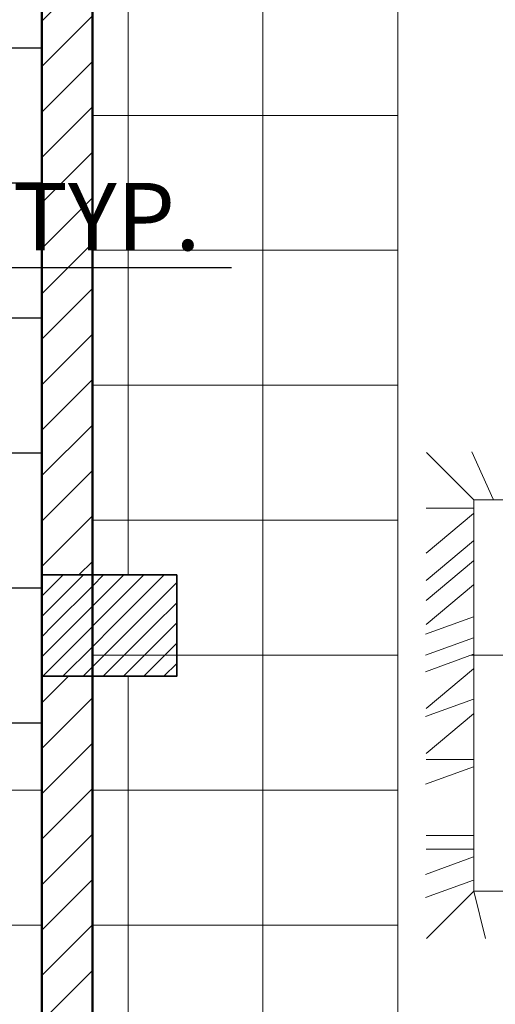
# Model space of a CAD drawing. Units: millimetres. Extents: x 225995 to 227247, y 225507 to 226008.
# Tile 5 of 23: x 226378 to 226421, y 225780 to 225867. Entities that reach past the tile are written whole.
import ezdxf

# ---------------------------------------------------------------- set-up
doc = ezdxf.new("R2010")
doc.units = ezdxf.units.MM
for name, color, linetype, lineweight in [('A-ANNO-DIMS', 2, 'Continuous', 18), ('A-COLS', 40, 'Continuous', 35), ('A-FLOR-PATT', 8, 'Continuous', 13), ('A-FLOR-STRS', 141, 'Continuous', 25), ('A-FURN', 9, 'Continuous', 18), ('A-WALL', 7, 'Continuous', 50), ('A-WALL-PATT', 8, 'Continuous', 13)]:
    doc.layers.add(name, color=color, linetype=linetype, lineweight=lineweight)
doc.styles.get("Standard").update_dxf_attribs({"font": 'arial.ttf'})
doc.dimstyles.new('ISO-25', dxfattribs={"dimtxt": 6, "dimasz": 2.5, "dimexe": 1.25, "dimexo": 0.625, "dimtad": 1, "dimdec": 0, "dimlunit": 3, "dimtxsty": 'Standard', "dimcen": 2.5, "dimadec": 0, "dimazin": 0, "dimtfac": 1, "dimtdec": 0, "dimtmove": 0, "dimatfit": 3, "dimfxl": 1, "dimarcsym": 0})
pattern_1 = [(45, (0, 118.1362), (-0.898025612, 0.898025612), [])]

# ---------------------------------------------------------------- blocks, each defined once
blk = doc.blocks.new('A$C6D2A2628')
for p, q in [((0.1019, 0.9267), (0.0019, 1.0267)), ((0.0977, 1.0278), (0.1431, 0.9278)), ((0.291, 0.9267), (0.1019, 0.9267)), ((0.1019, 0.9267), (0.1019, 0.1)), ((0.0015, 0.9091), (0.1015, 0.9091)), ((0.0015, 0.8141), (0.1015, 0.8978)), ((0.0015, 0.7564), (0.1015, 0.84)), ((0.0015, 0.7139), (0.1015, 0.7975)), ((0.0015, 0.6633), (0.1015, 0.7469)), ((0, 0.6428), (0.1015, 0.6794)), ((0, 0.5984), (0.1015, 0.6351)), ((0, 0.5636), (0.1015, 0.6003)), ((0.0015, 0.4859), (0.1015, 0.5695)), ((0, 0.4686), (0.1015, 0.5053)), ((0.0015, 0.3909), (0.1015, 0.4745)), ((0.0015, 0.3783), (0.1015, 0.3783)), ((0, 0.3261), (0.1015, 0.3628)), ((0.0015, 0.2173), (0.1015, 0.2173)), ((0.0015, 0.1884), (0.1015, 0.1884)), ((0, 0.1355), (0.1015, 0.1722)), ((0, 0.0863), (0.1015, 0.1229)), ((0.1019, 0.1), (0.0019, 0)), ((0.1019, 0.1), (1.9932, 0.1)), ((0.1019, 0.1), (0.1266, 0))]:
    blk.add_line(p, q)
blk = doc.blocks.new('*D81')
at = {"layer": 'A-ANNO-DIMS', "color": 0, "lineweight": -2, "transparency": 16777216}
for p, q in [((226280.276, 225843.99), (226280.276, 225846.51)), ((226292.912, 225843.99), (226292.912, 225846.51)), ((226282.776, 225845.26), (226290.412, 225845.26)), ((226292.912, 225845.26), (226397.254, 225845.26))]:
    blk.add_line(p, q, dxfattribs=at)
at = {"layer": 'A-ANNO-DIMS', "color": 0, "transparency": 16777216}
for points in [[(226282.776, 225845.677), (226282.776, 225844.844), (226280.276, 225845.26)], [(226290.412, 225845.677), (226290.412, 225844.844), (226292.912, 225845.26)]]:
    blk.add_solid(points, dxfattribs=at)
at = {"layer": 'Defpoints', "color": 0, "transparency": 16777216}
for p in [(226292.912, 225845.26), (226280.276, 225843.365), (226292.912, 225843.365)]:
    blk.add_point(p, dxfattribs=at)
at = {"layer": 'A-ANNO-DIMS', "color": 0, "transparency": 16777216, "insert": (226346.333, 225848.99), "char_height": 6, "attachment_point": 5}
blk.add_mtext('BAR STOOL 1\'-0 1/2" TYP.', dxfattribs=at)

msp = doc.modelspace()

# ---------------------------------------------------------------- hatches: boundary and pattern name
at = {"layer": 'A-WALL-PATT'}
h = msp.add_hatch(dxfattribs=at)
h.set_pattern_fill('ANSI31', color=256, scale=0.9)
h.paths.add_polyline_path([(226384.876, 225924.774), (226380.376, 225924.774), (226380.376, 225817.91), (226384.876, 225817.91)])
h = msp.add_hatch(dxfattribs=at)
h.set_pattern_fill('ANSI31', color=256, scale=0.4)
h.set_pattern_definition(pattern_1)
h.paths.add_polyline_path([(226384.876, 225817.91), (226380.376, 225817.91), (226380.376, 225813.41), (226384.876, 225813.41)])
h = msp.add_hatch(dxfattribs=at)
h.set_pattern_fill('ANSI31', color=256, scale=0.4)
h.set_pattern_definition(pattern_1)
h.paths.add_polyline_path([(226392.376, 225817.91), (226384.876, 225817.91), (226384.876, 225813.41), (226392.376, 225813.41)])
h = msp.add_hatch(dxfattribs=at)
h.set_pattern_fill('ANSI31', color=256, scale=0.4)
h.set_pattern_definition(pattern_1)
h.paths.add_polyline_path([(226384.876, 225813.41), (226380.376, 225813.41), (226380.376, 225808.91), (226384.876, 225808.91)])
h = msp.add_hatch(dxfattribs=at)
h.set_pattern_fill('ANSI31', color=256, scale=0.4)
h.set_pattern_definition(pattern_1)
h.paths.add_polyline_path([(226392.376, 225813.41), (226384.876, 225813.41), (226384.876, 225808.91), (226392.376, 225808.91)])
h = msp.add_hatch(dxfattribs=at)
h.set_pattern_fill('ANSI31', color=256, scale=0.9)
h.paths.add_polyline_path([(226384.876, 225808.91), (226380.376, 225808.91), (226380.376, 225740.274), (226384.876, 225740.274)])

# ---------------------------------------------------------------- linework, layer by layer
at = {"layer": 'A-COLS'}
msp.add_lwpolyline([(226380.376, 225808.91), (226380.376, 225817.91), (226392.376, 225817.91), (226392.376, 225808.91)], close=True, dxfattribs=at)
at = {"layer": 'A-FLOR-PATT'}
for p, q in [((226388.047, 225900.774), (226388.047, 225817.91)), ((226400.047, 225900.774), (226400.047, 225695.274)), ((226412.047, 225900.774), (226412.047, 225695.274)), ((226384.876, 225858.774), (226412.047, 225858.774)), ((226384.876, 225846.774), (226412.047, 225846.774)), ((226384.876, 225834.774), (226412.047, 225834.774)), ((226384.876, 225822.774), (226412.047, 225822.774)), ((226384.876, 225810.774), (226412.047, 225810.774)), ((226418.553, 225810.774), (226426.755, 225810.774)), ((226388.047, 225808.91), (226388.047, 225699.774)), ((226219.876, 225798.774), (226380.376, 225798.774)), ((226384.876, 225798.774), (226412.047, 225798.774)), ((226219.876, 225786.774), (226380.376, 225786.774)), ((226384.876, 225786.774), (226412.047, 225786.774))]:
    msp.add_line(p, q, dxfattribs=at)
at = {"layer": 'A-FLOR-STRS'}
for p, q in [((226344.376, 225864.774), (226380.376, 225864.774)), ((226344.376, 225852.774), (226380.376, 225852.774)), ((226344.376, 225840.774), (226380.376, 225840.774)), ((226344.376, 225828.774), (226380.376, 225828.774)), ((226344.376, 225816.774), (226380.376, 225816.774)), ((226338.376, 225804.774), (226380.376, 225804.774))]:
    msp.add_line(p, q, dxfattribs=at)
at = {"layer": 'A-WALL'}
for p, q in [((226380.376, 225740.274), (226380.376, 225924.774)), ((226380.376, 225924.774), (226380.376, 225740.274)), ((226384.876, 225740.274), (226384.876, 225924.774)), ((226384.876, 225740.274), (226384.876, 225924.774))]:
    msp.add_line(p, q, dxfattribs=at)

# ---------------------------------------------------------------- block references
at = {"layer": 'A-FURN', "xscale": 42.09102840542158, "yscale": 42.09102840542158, "zscale": 42.09102840542158}
msp.add_blockref('A$C6D2A2628', (226414.508, 225785.589), dxfattribs=at)

# ---------------------------------------------------------------- dimensions: what is measured, and where the dimension line sits
at = {"layer": 'A-ANNO-DIMS'}
dim = msp.add_linear_dim(base=(226292.912, 225845.26), p1=(226280.276, 225843.365), p2=(226292.912, 225843.365), text='BAR STOOL <> TYP.', dimstyle='ISO-25', override={"dimdec": 1, "dimrnd": 0, "dimzin": 1, "dimlunit": 4, "dimfrac": 2}, dxfattribs=at)
dim.commit()
dim.dimension.update_dxf_attribs({"geometry": '*D81', "text_midpoint": (226346.333, 225848.99)})

doc.saveas('drawing.dxf')
